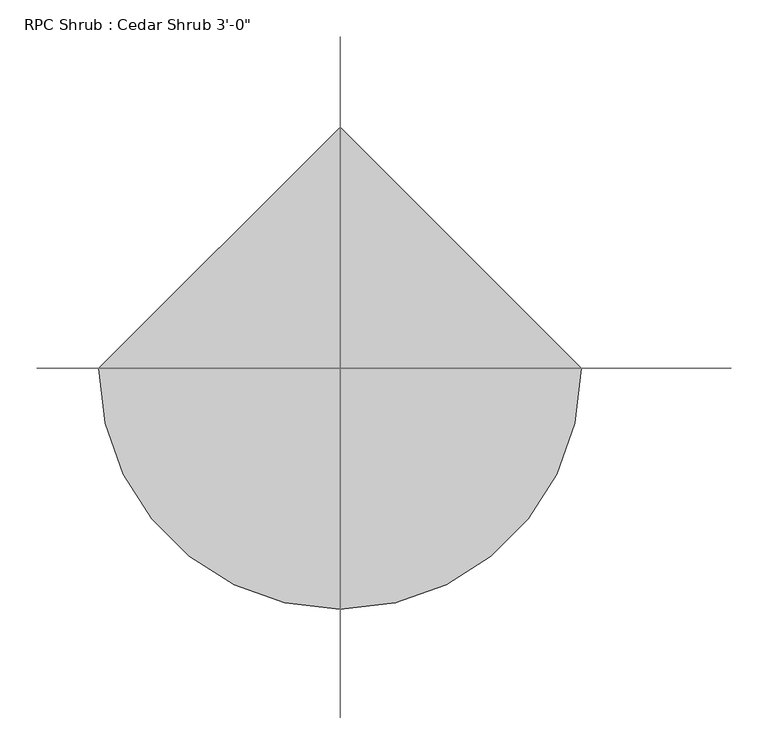
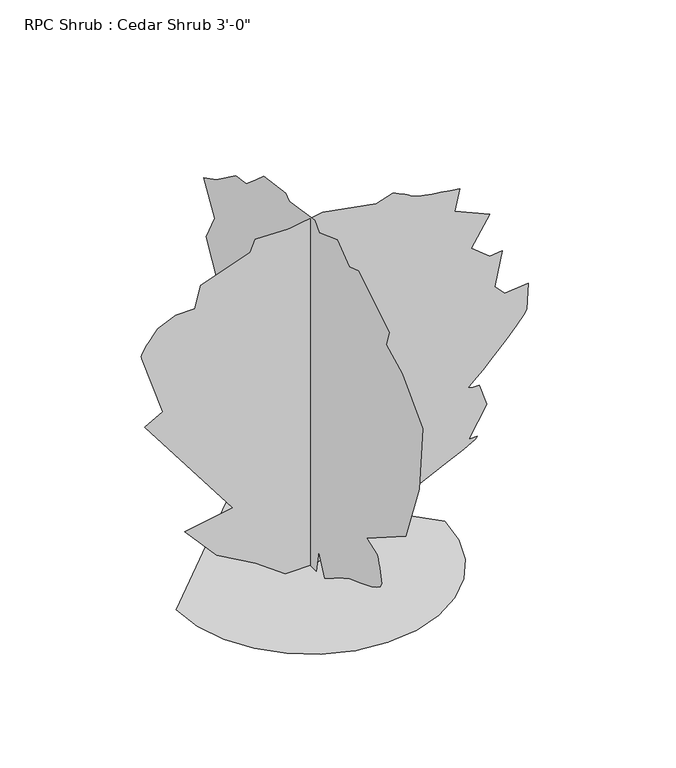
"""IFC4 building model written with IfcOpenShell, lengths in millimetres: geographic element geometry."""

from ifc_helpers import new_model, si_unit, origin, place, context, project, spatial, triangles, source, transform, mapped, element, save


def geographic_element_e27c54a3(model_context):
    return source(origin(), model_context, "Body", "Tessellation", [
        triangles([(-61.9491257, 8.98e-05, 3.1e-06), (-133.3686489, 8.41e-05, 52.0161927), (-229.784339, 7.75e-05, 107.3658847), (-308.3460772, 6.7e-05, 194.8542219), (-190.5039605, 6.45e-05, 216.2798944), (-406.5450977, 3.06e-05, 500.1695792), (-361.9096318, 2.77e-05, 525.1682714), (-413.687576, 9.1e-06, 680.504611), (-414.3708555, 8.5e-06, 686.0316719), (-412.1483531, 7.6e-06, 693.2453304), (-407.5052135, 6.6e-06, 701.8660252), (-400.9240746, 5.4e-06, 711.6120146), (-392.892588, 4.2e-06, 722.1987957), (-383.8933554, 2.8e-06, 733.3493505), (-374.4090142, 1.5e-06, 744.7793941), (-329.7710049, -9e-07, 764.4212185), (-283.347385, -9e-07, 764.4212185), (-269.0649538, -7.7e-06, 821.5560305), (-147.6523519, -1.28e-05, 864.4084293), (-135.1542685, -1.62e-05, 892.975799), (-51.2369207, -1.6e-05, 891.1902248), (30.8950596, -1.77e-05, 905.4726379), (161.2347623, -1.49e-05, 882.2620634), (202.3007514, -1.64e-05, 894.7614458), (209.926594, -1.6e-05, 891.3197227), (217.3964869, -1.56e-05, 887.8932604), (224.5539534, -1.52e-05, 884.4998629), (231.2430618, -1.48e-05, 881.1521021), (237.3073174, -1.44e-05, 877.8678549), (242.5910246, -1.4e-05, 874.6623819), (246.9374708, -1.36e-05, 871.5483278), (253.4703569, -1.33e-05, 868.4368898), (264.8764921, -1.29e-05, 865.2288008), (280.3400286, -1.25e-05, 861.9446262), (299.0547657, -1.21e-05, 858.5968655), (320.205346, -1.17e-05, 855.2034679), (342.9790286, -1.13e-05, 851.779549), (366.5654886, -1.09e-05, 848.337826), (354.0661062, -4.5e-06, 794.774235), (439.7683242, 0.0, 757.2787766), (395.1328583, 8.7e-06, 684.0733612), (439.7683242, 1.3e-05, 648.3660204), (470.1213407, 1.25e-05, 651.9346979), (452.2676702, 2.3e-05, 564.4468695), (477.2638553, 2.59e-05, 539.4507208), (534.3986309, 2.53e-05, 544.8075886), (530.8274099, 3.32e-05, 478.7446515), (523.5757087, 3.45e-05, 467.3451293), (504.7390314, 3.72e-05, 445.2623566), (478.6837177, 4.06e-05, 416.9032228), (449.7886428, 4.42e-05, 386.6696031), (422.4251967, 4.75e-05, 358.9657708), (400.96219, 4.99e-05, 338.196181), (389.7760268, 5.11e-05, 328.7651796), (386.8499336, 5.13e-05, 326.7306381), (386.9235847, 5.15e-05, 325.1634373), (389.4940673, 5.16e-05, 323.9874189), (394.0660629, 5.17e-05, 323.1212654), (400.1341518, 5.18e-05, 322.491362), (407.2029791, 5.19e-05, 322.0189344), (414.7721755, 5.19e-05, 321.622665), (432.6258459, 5.85e-05, 266.2734999), (387.99038, 6.75e-05, 191.2832371), (409.4153077, 6.75e-05, 191.2832371), (404.6121489, 6.81e-05, 185.7135189), (376.0066638, 7e-05, 170.1179047), (327.5713572, 7.28e-05, 146.167468), (263.2661253, 7.65e-05, 115.5335185), (187.0642904, 8.07e-05, 79.8863666), (102.9282468, 8.54e-05, 40.8973356), (14.7802468, 9.02e-05, 3.1e-06), (0.000381, 25.9026863, 6.2e-06), (0.0459126, 34.8300324, 57.3728062), (0.0459011, 134.816453, 119.8644768), (0.045878, 290.1520569, 198.4252067), (0.0458666, 418.7066374, 332.3364006), (0.0458549, 445.4884329, 412.6817508), (0.0458666, 354.4293471, 416.2530081), (0.0458666, 391.9248419, 493.0296444), (0.0458549, 441.9171756, 584.0886938), (0.0458549, 406.2098348, 653.7203447), (0.0458549, 452.6309112, 730.496981), (0.0458549, 400.852967, 757.2787766), (0.0458666, 316.9338161, 817.9848095), (0.0458666, 272.2983865, 825.1272514), (0.0458666, 229.4465145, 860.8371357), (0.045878, 197.3081237, 889.404578), (0.045878, 104.4634274, 901.901417), (0.045878, 90.1794701, 889.404578), (0.0458895, -18.7343943, 907.2582121), (0.0459011, -38.3746062, 885.833357), (0.0459011, -115.1499754, 914.4007267), (0.0459126, -165.1433174, 875.1196215), (0.0459126, -202.6383216, 887.6189312), (0.0459357, -334.7646317, 807.2710739), (0.0459357, -322.2652857, 767.9924395), (0.0459357, -390.1138332, 734.068202), (0.0459474, -477.6016617, 644.7947268), (0.0459588, -463.3167051, 478.7446515), (0.0459474, -404.3962463, 321.622665), (0.0459357, -240.1333076, 216.2798944), (0.0459474, -284.7697909, 200.2108353), (0.0459474, -287.8203315, 191.0282199), (0.0459474, -290.8073766, 181.8458589), (0.0459474, -293.6724997, 172.6634979), (0.0459474, -296.3471184, 163.4808825), (0.0459474, -298.7728243, 154.2985215), (0.0459474, -300.8861037, 145.1161604), (0.0459474, -302.6260048, 135.9335451), (0.0459474, -297.7517384, 125.9028165), (0.0459474, -282.4482212, 114.7161447), (0.0459474, -260.2740114, 103.1860617), (0.0459357, -234.7871223, 92.1246003), (0.0459357, -209.5511809, 82.3433114), (0.0459357, -188.1255083, 74.6549771), (0.0459357, -174.0706613, 69.8711394), (0.0459357, -161.0932739, 63.9628381), (0.0459357, -142.4006376, 53.6509403), (0.0459357, -120.8030006, 40.8714288), (0.0459243, -99.1118918, 27.5610539), (0.0459243, -80.1380772, 15.6561154), (0.0459243, -66.6923272, 7.0931586), (0.0459243, -61.5856531, 3.8085299), (0.0459243, -36.5889844, 59.1581714), (0.0003925, -25.8762707, 0.0), (-329.2655488, 0.0, 9.54e-05), (-320.5609566, -75.445681, 8.64e-05), (-295.7705366, -144.7305826, 7.82e-05), (-256.8780341, -205.8697014, 0.0001171), (-205.8697014, -256.8780341, 0.000111), (-144.7305826, -295.7705366, 0.0001064), (-75.445681, -320.5609566, 0.0001034), (1.15e-05, -329.2655488, 0.0001024), (75.4459354, -320.5609566, 0.0001034), (144.7305826, -295.7705366, 0.0001064), (205.8697014, -256.8780341, 0.000111), (256.8780341, -205.8697014, 0.0001171), (295.7705366, -144.7305826, 7.82e-05), (320.5609566, -75.445681, 8.64e-05), (329.2655488, 2.88e-05, 9.54e-05), (-4.62e-05, 329.2655488, 8.85e-05)], [[63, 64, 65], [63, 65, 66], [3, 4, 5], [42, 43, 44], [45, 46, 47], [5, 6, 7], [39, 40, 41], [37, 38, 39], [2, 3, 5], [45, 47, 48], [45, 48, 49], [36, 37, 39], [60, 61, 62], [19, 20, 21], [59, 60, 62], [59, 62, 63], [58, 59, 63], [57, 58, 63], [56, 57, 63], [45, 49, 50], [17, 18, 19], [35, 36, 39], [45, 50, 51], [44, 45, 51], [44, 51, 52], [41, 42, 44], [23, 24, 25], [34, 35, 39], [44, 52, 53], [41, 44, 53], [41, 53, 54], [41, 54, 55], [1, 2, 5], [71, 1, 5], [70, 71, 5], [69, 70, 5], [68, 69, 5], [68, 5, 7], [67, 68, 7], [66, 67, 7], [63, 66, 7], [56, 63, 7], [55, 56, 7], [41, 55, 7], [39, 41, 7], [34, 39, 7], [33, 34, 7], [32, 33, 7], [31, 32, 7], [30, 31, 7], [29, 30, 7], [28, 29, 7], [27, 28, 7], [26, 27, 7], [25, 26, 7], [23, 25, 7], [22, 23, 7], [21, 22, 7], [19, 21, 7], [17, 19, 7], [17, 7, 8], [16, 17, 8], [15, 16, 8], [14, 15, 8], [13, 14, 8], [12, 13, 8], [11, 12, 8], [10, 11, 8], [9, 10, 8], [76, 77, 78], [122, 123, 124], [81, 82, 83], [121, 122, 124], [124, 125, 72], [124, 72, 73], [75, 76, 78], [120, 121, 124], [94, 95, 96], [93, 94, 96], [91, 92, 93], [119, 120, 124], [89, 90, 91], [79, 80, 81], [101, 102, 103], [81, 83, 84], [81, 84, 85], [97, 98, 99], [87, 88, 89], [96, 97, 99], [74, 75, 78], [96, 99, 100], [96, 100, 101], [93, 96, 101], [91, 93, 101], [89, 91, 101], [87, 89, 101], [86, 87, 101], [85, 86, 101], [81, 85, 101], [79, 81, 101], [78, 79, 101], [74, 78, 101], [73, 74, 101], [124, 73, 101], [119, 124, 101], [118, 119, 101], [117, 118, 101], [116, 117, 101], [115, 116, 101], [114, 115, 101], [113, 114, 101], [112, 113, 101], [112, 101, 103], [112, 103, 104], [112, 104, 105], [111, 112, 105], [111, 105, 106], [111, 106, 107], [110, 111, 107], [110, 107, 108], [109, 110, 108], [140, 141, 126], [139, 140, 126], [139, 126, 127], [138, 139, 127], [138, 127, 128], [138, 128, 129], [137, 138, 129], [136, 137, 129], [136, 129, 130], [136, 130, 131], [136, 131, 132], [136, 132, 133], [136, 133, 134], [136, 134, 135]], closed=False),
    ])


if __name__ == "__main__":
    model = new_model("IFC4")
    model_context = context("Model", 3, world=origin())
    ifc_project = project(units=[si_unit("LENGTHUNIT", "METRE", prefix="MILLI")], contexts=[model_context])
    site = spatial("IfcSite", under=ifc_project)
    building = spatial("IfcBuilding", under=site)
    placement = place(None, origin())
    geographic_element_shape = geographic_element_e27c54a3(model_context)
    element("IfcGeographicElement", 1, ObjectType="RPC Shrub : Cedar Shrub 3'-0\"", at=placement, inside=building, context=model_context, shape_type="MappedRepresentation", body=[
        mapped(geographic_element_shape, transform((0.0, 0.0, 0.0), x_axis=(1.0, 0.0, 0.0), y_axis=(0.0, 1.0, 0.0), z_axis=(0.0, 0.0, 1.0))),
    ])
    save(model, "model.ifc")

# Revit data of these elements
# Type "RPC Shrub : Cedar Shrub 3'-0\""
#   Type Comments = "Cedar Shrub"
#   built-in parameter 1005198 = "{2, 15},{39, RPC-16-FUMD-ULXX-U7X6-J000-ST1L-LVER-AU},{1, 0},{1, 0},{2, 13},{1, 8},{5, Color},{1, 0},{1, 0},{3, 0.8},{3, 0.8},{3, 0.8},{1, 8},{7, BBoxMin},{1, 0},{1, 0},{1, 0},{1, 0},{1, 0},{1, 8},{7, BBoxMax},{1, 0},{1, 0},{1, 0},{1, 0},{1, 0},{2, 11},{9, RPCTypeId},{1, 0},{1, 0},{39, RPC-16-FUMD-ULXX-U7X6-J000-ST1L-LVER-AU},{1, 6},{14, RPCPlantHeight},{1, 0},{1, 0},{1, 3},{2, 11},{7, keyword},{1, 0},{1, 0},{35, :RPCs:Shrubs [General]:Geometry:RPC},{2, 11},{8, category},{1, 0},{1, 0},{16, Shrubs [General]},{2, 11},{12, LocalizedUID},{1, 0},{1, 0},{11, Cedar Shrub},{2, 14},{6, Height},{1, 0},{1, 0},{1, 3},{1, 2},{16, Cast Reflections},{1, 0},{1, 0},{1, 0},{1, 2},{12, Cast Shadows},{1, 0},{1, 0},{1, 1},{1, 2},{9, Lock View},{1, 0},{1, 0},{1, 0},{1, 4},{5, ViewC},{1, 0},{1, 0},{1, 0},{21, assetlibrary_base.fbx},{1, 5},"
#   built-in parameter 1005195 = "RPC-16-FUMD-ULXX-U7X6-J000-ST1L-LVER-AU"
#   Assembly Code = "G2050500"
#   Height = 3' - 0"
#   Default Elevation = 0
